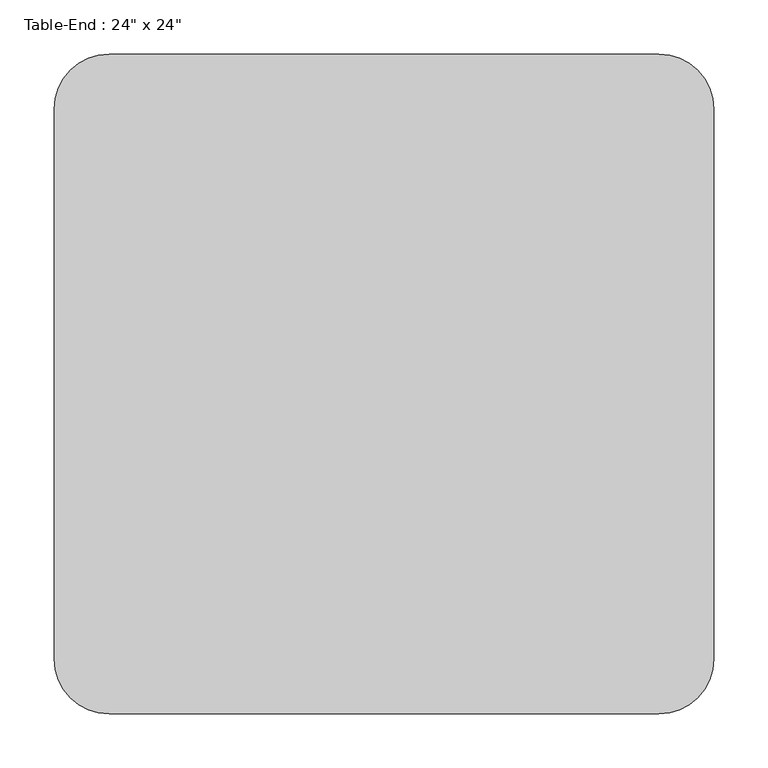
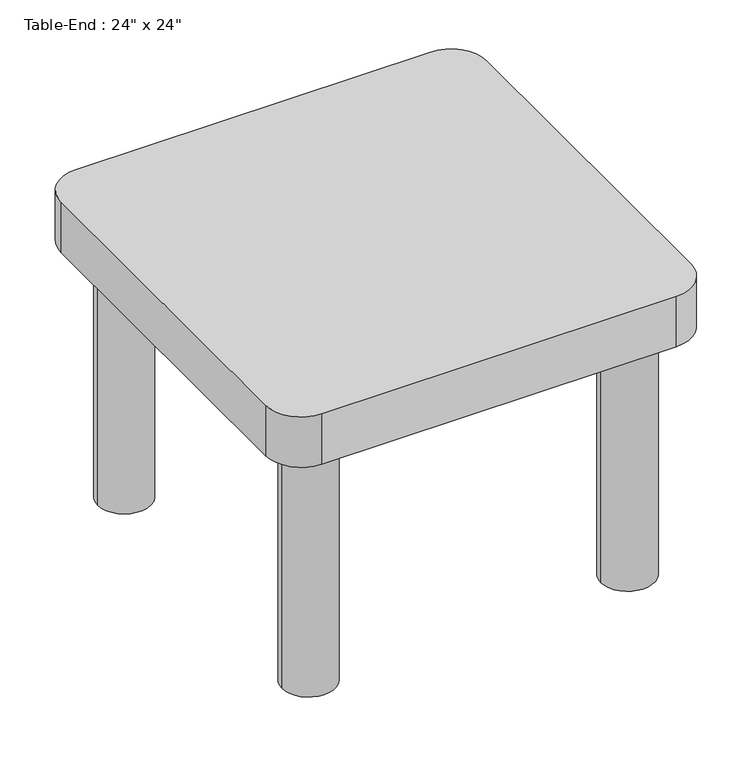
"""IFC4 building model written with IfcOpenShell, lengths in millimetres: furniture geometry."""

from ifc_helpers import new_model, si_unit, point, frame, frame_2d, origin, origin_with_axes, place, context, project, spatial, polyline, circle_curve, trimmed, segment, composite_curve, outline, extrude, source, transform, mapped, element, save


def furniture_5d68651d(model_context):
    return source(origin(), model_context, "Body", "SweptSolid", [
        extrude(outline(composite_curve([segment(polyline([(562.5336303, -152.4), (54.5336303, -152.4)]), True, "CONTINUOUS"), segment(trimmed(circle_curve(frame_2d((54.5336303, -101.6)), 50.8), [point((54.5336303, -152.4))], [point((3.7336303, -101.6))], False, "CARTESIAN"), True, "CONTINUOUS"), segment(polyline([(3.7336303, -101.6), (3.7336303, 406.4)]), True, "CONTINUOUS"), segment(trimmed(circle_curve(frame_2d((54.5336303, 406.4)), 50.8), [point((3.7336303, 406.4))], [point((54.5336303, 457.2))], False, "CARTESIAN"), True, "CONTINUOUS"), segment(polyline([(54.5336303, 457.2), (562.5336303, 457.2)]), True, "CONTINUOUS"), segment(trimmed(circle_curve(frame_2d((562.5336303, 406.4)), 50.8), [point((562.5336303, 457.2))], [point((613.3336303, 406.4))], False, "CARTESIAN"), True, "CONTINUOUS"), segment(polyline([(613.3336303, 406.4), (613.3336303, -101.6)]), True, "CONTINUOUS"), segment(trimmed(circle_curve(frame_2d((562.5336303, -101.6)), 50.8), [point((613.3336303, -101.6))], [point((562.5336303, -152.4))], False, "CARTESIAN"), True, "CONTINUOUS")], self_intersect=False)), frame((0.0, 0.0, 381.0), z_axis=(0.0, 0.0, 1.0), x_axis=(1.0, 0.0, 0.0)), (0.0, 0.0, 1.0), 76.2),
        extrude(outline(composite_curve([segment(trimmed(circle_curve(frame_2d((79.9336303, 381.0)), 38.1), [point((41.8336303, 381.0))], [point((118.0336303, 381.0))], False, "CARTESIAN"), True, "CONTINUOUS"), segment(trimmed(circle_curve(frame_2d((79.9336303, 381.0)), 38.1), [point((118.0336303, 381.0))], [point((41.8336303, 381.0))], False, "CARTESIAN"), True, "CONTINUOUS")], self_intersect=False)), origin_with_axes(), (0.0, 0.0, 1.0), 381.0),
        extrude(outline(composite_curve([segment(trimmed(circle_curve(frame_2d((79.9336303, -76.2)), 38.1), [point((41.8336303, -76.2))], [point((118.0336303, -76.2))], False, "CARTESIAN"), True, "CONTINUOUS"), segment(trimmed(circle_curve(frame_2d((79.9336303, -76.2)), 38.1), [point((118.0336303, -76.2))], [point((41.8336303, -76.2))], False, "CARTESIAN"), True, "CONTINUOUS")], self_intersect=False)), origin_with_axes(), (0.0, 0.0, 1.0), 381.0),
        extrude(outline(composite_curve([segment(trimmed(circle_curve(frame_2d((537.1336303, -76.2)), 38.1), [point((499.0336303, -76.2))], [point((575.2336303, -76.2))], False, "CARTESIAN"), True, "CONTINUOUS"), segment(trimmed(circle_curve(frame_2d((537.1336303, -76.2)), 38.1), [point((575.2336303, -76.2))], [point((499.0336303, -76.2))], False, "CARTESIAN"), True, "CONTINUOUS")], self_intersect=False)), origin_with_axes(), (0.0, 0.0, 1.0), 381.0),
        extrude(outline(composite_curve([segment(trimmed(circle_curve(frame_2d((537.1336303, 381.0)), 38.1), [point((499.0336303, 381.0))], [point((575.2336303, 381.0))], False, "CARTESIAN"), True, "CONTINUOUS"), segment(trimmed(circle_curve(frame_2d((537.1336303, 381.0)), 38.1), [point((575.2336303, 381.0))], [point((499.0336303, 381.0))], False, "CARTESIAN"), True, "CONTINUOUS")], self_intersect=False)), origin_with_axes(), (0.0, 0.0, 1.0), 381.0),
    ])


if __name__ == "__main__":
    model = new_model("IFC4")
    model_context = context("Model", 3, world=origin())
    ifc_project = project(units=[si_unit("LENGTHUNIT", "METRE", prefix="MILLI")], contexts=[model_context])
    site = spatial("IfcSite", under=ifc_project)
    building = spatial("IfcBuilding", under=site)
    placement = place(None, origin())
    furniture_shape = furniture_5d68651d(model_context)
    element("IfcFurniture", 1, ObjectType="Table-End : 24\" x 24\"", at=placement, inside=building, context=model_context, shape_type="MappedRepresentation", body=[
        mapped(furniture_shape, transform((0.0, 0.0, 0.0), x_axis=(1.0, 0.0, 0.0), y_axis=(0.0, 1.0, 0.0), z_axis=(0.0, 0.0, 1.0))),
    ])
    save(model, "model.ifc")

# Revit data of these elements
# Type "Table-End : 24\" x 24\""
#   Assembly Code = "E2020200"
#   Height = 1' - 6"
#   Length = 2' - 0"
#   Width = 2' - 0"
#   Base Material = Birch
#   Top Material = Laminate, Ivory, Matte
#   Default Elevation = 0
# Element 1 (IfcFurniture, "Table-End : 24\" x 24\"")
#   Materials on its faces: "Laminate, Ivory, Matte", "Birch"
# Materials
#   "Birch": class "Wood", colour RGB 224 178 126, transparency 0, Description = "Betula Alleghaniensis", Cost = 0
#   "Laminate, Ivory, Matte": class "Plastic", colour RGB 247 247 239, transparency 0, Description = "Plastic Laminate - Ivory, Matte", Cost = 0
